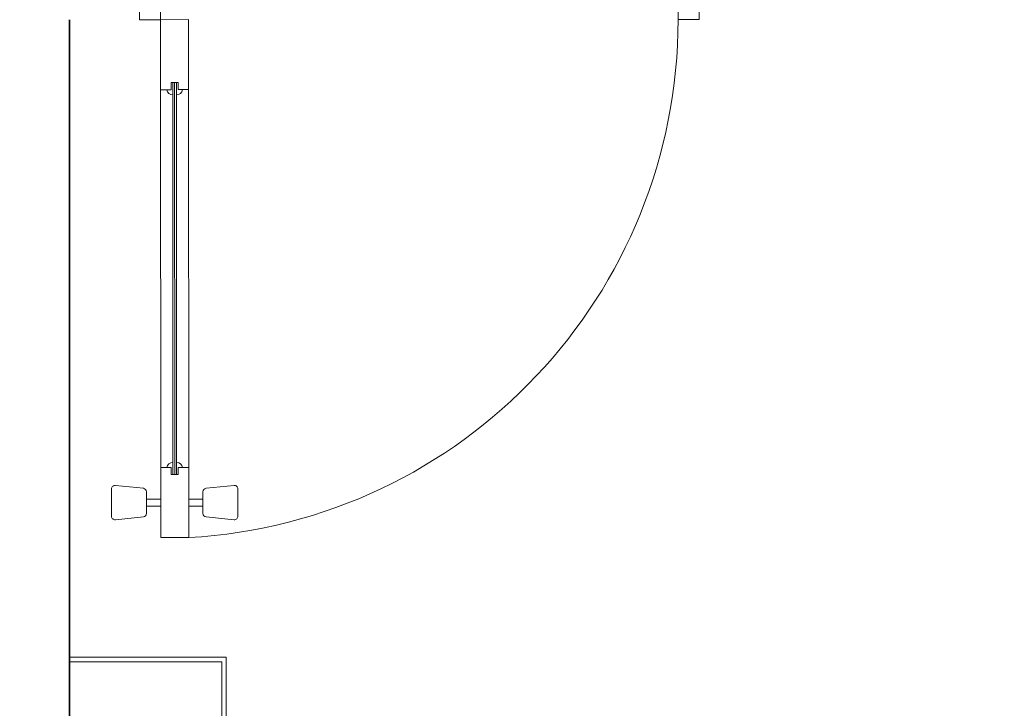
# Model space of a CAD drawing. Units: inches. Extents: x -638 to 186, y -762 to 59.
# Tile 11 of 31: x -164 to -100, y -457 to -413. Entities that reach past the tile are written whole.
import ezdxf

# ---------------------------------------------------------------- set-up
doc = ezdxf.new("R2010")
doc.units = ezdxf.units.IN
for name, color, linetype, lineweight in [('A-ANNO-DIMS', 2, 'Continuous', 18), ('A-DOOR', 3, 'Continuous', 18), ('furn', 8, 'Continuous', 13), ('wall', 7, 'Continuous', 35)]:
    doc.layers.add(name, color=color, linetype=linetype, lineweight=lineweight)
doc.styles.get("Standard").update_dxf_attribs({"font": 'arial.ttf'})
doc.dimstyles.new('ISO-25', dxfattribs={"dimtxt": 4, "dimasz": 4, "dimexe": 1.25, "dimexo": 0.625, "dimtad": 0, "dimlunit": 4, "dimtxsty": 'Standard', "dimcen": 2.5, "dimclrt": 256, "dimadec": 0, "dimazin": 0, "dimtfac": 1, "dimtmove": 0, "dimatfit": 3, "dimfxl": 1, "dimfxlon": 1, "dimarcsym": 0})

# ---------------------------------------------------------------- blocks, each defined once
blk = doc.blocks.new('DOOR-SWING-36IN')
for p, q in [((35.541, 35.096), (4.054, 35.086)), ((3.952, 4.049), (3.944, 29.238)), ((4.064, 4.049), (4.056, 29.238)), ((4.177, 4.049), (4.169, 29.238)), ((3.164, 4.498), (3.157, 28.788)), ((4.964, 4.499), (4.956, 28.789))]:
    blk.add_line(p, q)
for points in [[(3.155, 33.286), (3.155, 35.086), (4.054, 35.086), (4.053, 37.785), (1.804, 37.784), (1.806, 33.286), (3.155, 33.286)], [(36.442, 33.297), (36.441, 35.096), (35.541, 35.096), (35.541, 37.795), (37.79, 37.795), (37.791, 33.297), (36.442, 33.297)], [(4.281, 28.789), (4.956, 28.789), (4.955, 33.287), (3.155, 33.286), (3.157, 28.788), (3.831, 28.788), (3.831, 29.238), (4.281, 29.238), (4.281, 28.789)], [(4.289, 4.499), (4.964, 4.499), (4.965, 0.001), (3.166, 0), (3.164, 4.498), (3.839, 4.498), (3.839, 4.049), (4.289, 4.049), (4.289, 4.499)]]:
    blk.add_lwpolyline(points)
for points in [[(2.047, 3.169), (0.247, 3.348, 0.443716), (0, 3.124), (0.001, 1.372, 0.443716), (0.248, 1.148), (2.047, 1.329, 0.385314), (2.25, 1.553), (2.249, 2.945, 0.385314)], [(6.082, 3.17), (7.881, 3.35, -0.443716), (8.129, 3.127), (8.129, 1.375, -0.443716), (7.882, 1.151), (6.083, 1.33, -0.385314), (5.88, 1.554), (5.88, 2.946, -0.385314)]]:
    blk.add_lwpolyline(points, format="xyb", close=True)
for points in [[(3.165, 2.474), (2.249, 2.474), (2.249, 2.024), (3.165, 2.024)], [(4.964, 2.475), (5.88, 2.475), (5.88, 2.025), (4.964, 2.025)]]:
    blk.add_lwpolyline(points, close=True)
for centre, radius, start, end in [((3.064, 33.324), 33.378, 273.26531, 359.95298), ((3.923, 28.83), 0.371, 186.45223, 273.3078), ((4.19, 28.83), 0.371, 266.72821, 353.58377), ((3.93, 4.457), 0.371, 86.72821, 173.58377), ((4.198, 4.457), 0.371, 6.45223, 93.3078)]:
    blk.add_arc(centre, radius, start, end)
blk = doc.blocks.new('BED-DOUBLE-WITH-NIGHTSTANDS')
for p, q in [((0, 59.951), (78.699, 59.951)), ((78.411, 50.162), (78.411, 59.951)), ((78.699, 49.874), (78.699, 59.951)), ((62.191, 50.162), (78.411, 50.162)), ((61.904, 49.874), (78.699, 49.874))]:
    blk.add_line(p, q)
blk = doc.blocks.new('*D38')
at = {"layer": 'A-ANNO-DIMS', "color": 0, "lineweight": -2, "transparency": 16777216}
for p, q in [((182.663, -280.533), (184.913, -280.533)), ((183.663, -284.533), (183.663, -371.726)), ((183.663, -473.533), (183.663, -386.34)), ((182.663, -477.533), (184.913, -477.533))]:
    blk.add_line(p, q, dxfattribs=at)
at = {"layer": 'A-ANNO-DIMS', "color": 0, "lineweight": 30, "transparency": 16777216}
for points in [[(182.997, -284.533), (184.33, -284.533), (183.663, -280.533)], [(182.997, -473.533), (184.33, -473.533), (183.663, -477.533)]]:
    blk.add_solid(points, dxfattribs=at)
at = {"layer": 'Defpoints', "color": 0, "lineweight": 30, "transparency": 16777216}
for p in [(-404.526, -280.533), (-404.526, -477.533), (183.663, -477.533)]:
    blk.add_point(p, dxfattribs=at)
at = {"layer": 'A-ANNO-DIMS', "transparency": 16777216, "insert": (183.663, -379.033), "char_height": 4, "attachment_point": 5, "rotation": 90}
blk.add_mtext('16\'-5"', dxfattribs=at)

msp = doc.modelspace()

# ---------------------------------------------------------------- linework, layer by layer
at = {"layer": 'wall'}
msp.add_line((-160.526, -412.533), (-160.526, -539.033), dxfattribs=at)

# ---------------------------------------------------------------- block references
at = {"layer": 'A-DOOR'}
msp.add_blockref('DOOR-SWING-36IN', (-157.83, -445.817), dxfattribs=at)
at = {"layer": 'furn', "rotation": 90.00000000000017}
msp.add_blockref('BED-DOUBLE-WITH-NIGHTSTANDS', (-100.575, -532.203), dxfattribs=at)

# ---------------------------------------------------------------- dimensions: what is measured, and where the dimension line sits
at = {"layer": 'A-ANNO-DIMS'}
dim = msp.add_linear_dim(base=(183.663, -477.533), p1=(-404.526, -280.533), p2=(-404.526, -477.533), angle=90, dimstyle='ISO-25', override={"dimdec": 1, "dimlfac": 1, "dimrnd": 0, "dimzin": 1, "dimdsep": 46, "dimlunit": 4, "dimfrac": 2}, dxfattribs=at)
dim.commit()
dim.dimension.update_dxf_attribs({"geometry": '*D38', "text_midpoint": (183.663, -379.033)})

doc.saveas('drawing.dxf')
